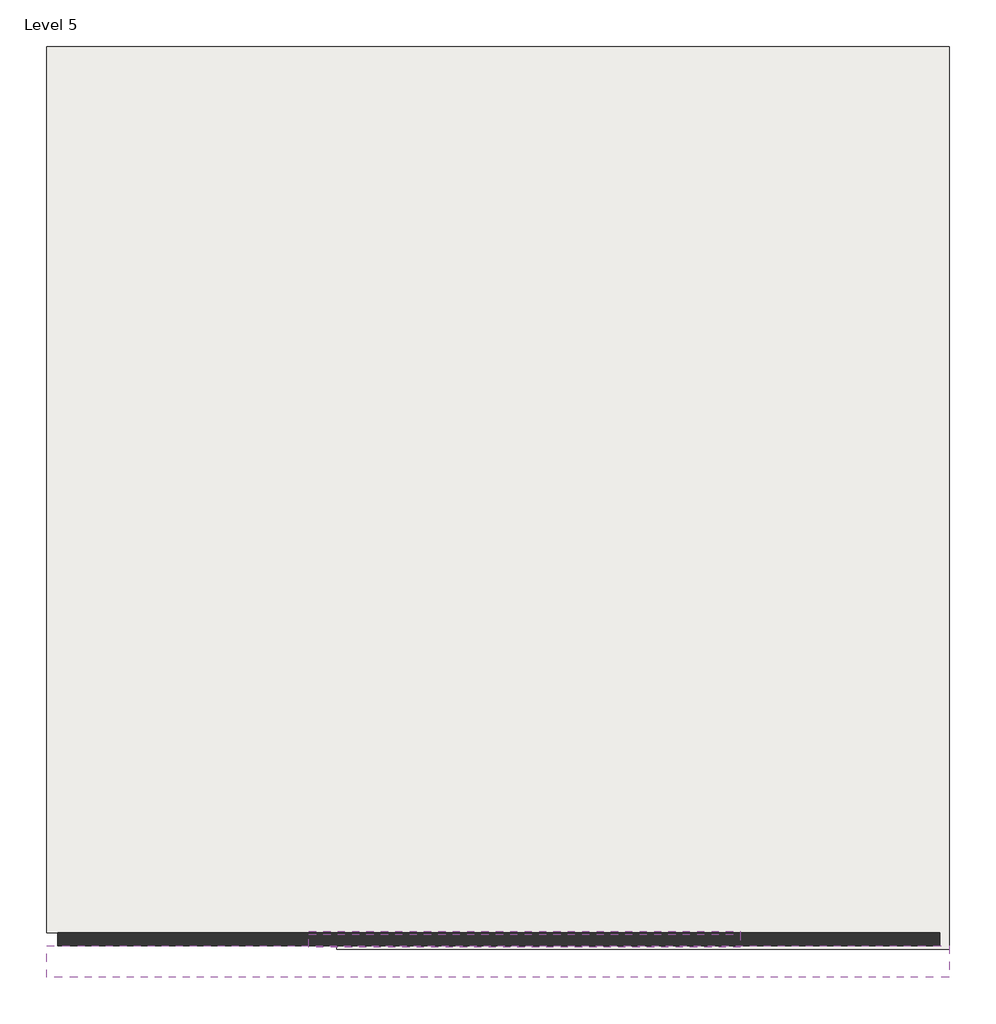
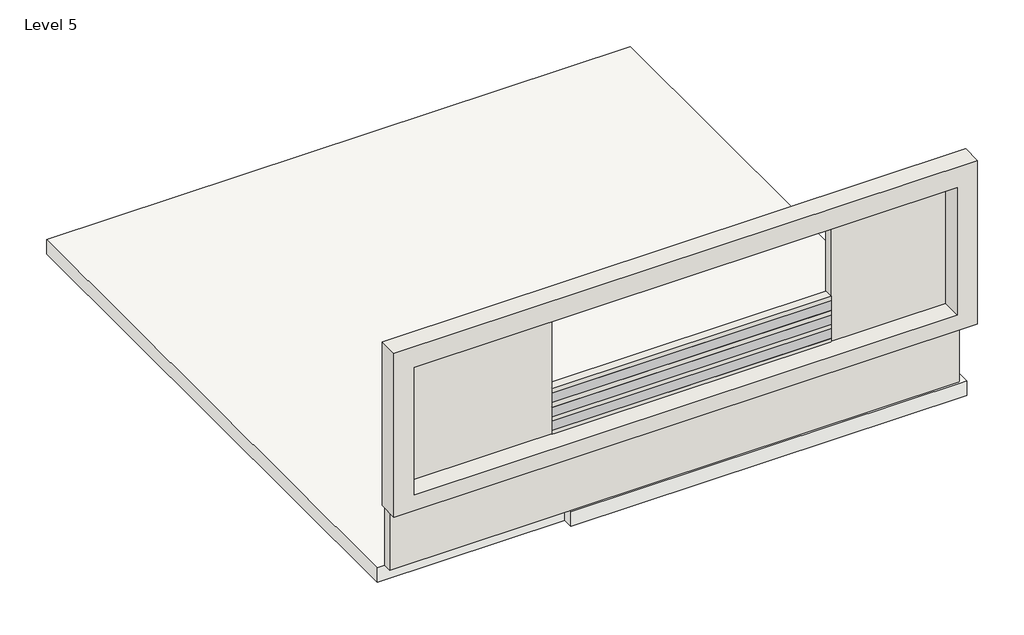
# One storey: 3 proxies, 3 walls, 1 roof.
"""IFC4 building model written with IfcOpenShell, lengths in millimetres."""

from ifc_helpers import new_model, si_unit, frame, origin, place, context, project, spatial, polyline, outline, extrude, faceted_brep, transform, mapped, element, save
from components import walls_4_walls_4_69c7fff0

model = new_model("IFC4")

# Units and contexts
model_context = context("Model", 3, world=origin())
ifc_project = project(units=[si_unit("LENGTHUNIT", "METRE", prefix="MILLI")], contexts=[model_context])

# Site, building, storey
site = spatial("IfcSite", under=ifc_project)
building = spatial("IfcBuilding", under=site)
storey = spatial("IfcBuildingStorey", under=building, Name="Level 5", Elevation=15544.8)

# Proxies
placement = place(None, origin())
element("IfcBuildingElementProxy", 1, Name="Reveal", ObjectType="Reveal", at=placement, inside=storey, context=model_context, shape_type="SweptSolid", body=[
    extrude(outline(polyline([(-6293.9561565, 1484.2485991), (-6293.9561565, 1636.6485991), (-2118.5901764, 1636.6485991), (-2118.5901764, 1484.2485991), (-6293.9561565, 1484.2485991)])), frame((0.0, 0.0, 17589.4520409), z_axis=(0.0, 0.0, 1.0), x_axis=(1.0, 0.0, 0.0)), (0.0, 0.0, 1.0), 152.4),
])
element("IfcBuildingElementProxy", 2, Name="Reveal", ObjectType="Reveal", at=placement, inside=storey, context=model_context, shape_type="SweptSolid", body=[
    extrude(outline(polyline([(-6293.9561565, 1484.2485991), (-6293.9561565, 1636.6485991), (-2118.5901764, 1636.6485991), (-2118.5901764, 1484.2485991), (-6293.9561565, 1484.2485991)])), frame((0.0, 0.0, 17360.8520409), z_axis=(0.0, 0.0, 1.0), x_axis=(1.0, 0.0, 0.0)), (0.0, 0.0, 1.0), 152.4),
])
element("IfcBuildingElementProxy", 3, Name="Reveal", ObjectType="Reveal", at=placement, inside=storey, context=model_context, shape_type="SweptSolid", body=[
    extrude(outline(polyline([(-6293.9561565, 1484.2485991), (-6293.9561565, 1636.6485991), (-2118.5901764, 1636.6485991), (-2118.5901764, 1484.2485991), (-6293.9561565, 1484.2485991)])), frame((0.0, 0.0, 17145.0), z_axis=(0.0, 0.0, 1.0), x_axis=(1.0, 0.0, 0.0)), (0.0, 0.0, 1.0), 152.4),
])

# Roof
element("IfcRoof", 4, ObjectType="Generic - 9\"", at=placement, inside=storey, context=model_context, shape_type="SweptSolid", body=[
    extrude(outline(polyline([(-8833.9561565, 10202.7985991), (-96.3561565, 10202.7985991), (-96.3561565, 1465.1985991), (-6027.2561565, 1465.1985991), (-6027.2561565, 1623.9485991), (-8833.9561565, 1623.9485991), (-8833.9561565, 10202.7985991)])), frame((0.0, 0.0, 15544.8), z_axis=(0.0, 0.0, 1.0), x_axis=(1.0, 0.0, 0.0)), (0.0, 0.0, 1.0), 228.6),
])

# Walls
element("IfcWall", 5, ObjectType="Generic - 5\"", at=placement, inside=storey, context=model_context, shape_type="Brep", body=[
    faceted_brep([(-8724.447025, 1496.6402851, 15773.4), (-190.047025, 1496.6402851, 15773.4), (-190.047025, 1496.6402851, 19202.4), (-2118.5901764, 1496.6402851, 19202.4), (-2118.5901764, 1496.6402851, 17741.8520409), (-2118.5901764, 1496.6402851, 17589.4520409), (-2118.5901764, 1496.6402851, 17513.2520409), (-2118.5901764, 1496.6402851, 17360.8520409), (-2118.5901764, 1496.6402851, 17297.4), (-2118.5901764, 1496.6402851, 17145.0), (-2118.5901764, 1496.6402851, 17087.4973119), (-6293.9561565, 1496.6402851, 17087.4973119), (-6293.9561565, 1496.6402851, 17145.0), (-6293.9561565, 1496.6402851, 17297.4), (-6293.9561565, 1496.6402851, 17360.8520409), (-6293.9561565, 1496.6402851, 17513.2520409), (-6293.9561565, 1496.6402851, 17589.4520409), (-6293.9561565, 1496.6402851, 17741.8520409), (-6293.9561565, 1496.6402851, 19202.4), (-8724.447025, 1496.6402851, 19202.4), (-190.047025, 1623.6402851, 15773.4), (-8724.447025, 1623.6402851, 15773.4), (-8724.447025, 1623.6402851, 19202.4), (-6293.9561565, 1623.6402851, 19202.4), (-6293.9561565, 1623.6402851, 17741.8520409), (-6293.9561565, 1623.6402851, 17589.4520409), (-6293.9561565, 1623.6402851, 17513.2520409), (-6293.9561565, 1623.6402851, 17360.8520409), (-6293.9561565, 1623.6402851, 17297.4), (-6293.9561565, 1623.6402851, 17145.0), (-6293.9561565, 1623.6402851, 17087.4973119), (-2118.5901764, 1623.6402851, 17087.4973119), (-2118.5901764, 1623.6402851, 17145.0), (-2118.5901764, 1623.6402851, 17297.4), (-2118.5901764, 1623.6402851, 17360.8520409), (-2118.5901764, 1623.6402851, 17513.2520409), (-2118.5901764, 1623.6402851, 17589.4520409), (-2118.5901764, 1623.6402851, 17741.8520409), (-2118.5901764, 1623.6402851, 19202.4), (-190.047025, 1623.6402851, 19202.4), (-2118.5901764, 1611.2485991, 17087.4973119), (-6293.9561565, 1611.2485991, 17087.4973119)], [[[0, 1, 2, 3, 4, 5, 6, 7, 8, 9, 10, 11, 12, 13, 14, 15, 16, 17, 18, 19]], [[20, 21, 22, 23, 24, 25, 26, 27, 28, 29, 30, 31, 32, 33, 34, 35, 36, 37, 38, 39]], [[1, 0, 21, 20]], [[2, 1, 20, 39]], [[0, 19, 22, 21]], [[3, 2, 39, 38]], [[3, 38, 37, 36, 35, 34, 33, 32, 31, 40, 10, 9, 8, 7, 6, 5, 4]], [[11, 10, 40, 31, 30, 41]], [[11, 41, 30, 29, 28, 27, 26, 25, 24, 23, 18, 17, 16, 15, 14, 13, 12]], [[19, 18, 23, 22]]]),
])
element("IfcWall", 6, ObjectType="Generic - 5\"", at=placement, inside=storey, context=model_context, shape_type="Brep", body=[
    faceted_brep([(-6293.9561565, 1484.2485991, 17087.4973119), (-2118.5901764, 1484.2485991, 17087.4973119), (-2118.5901764, 1484.2485991, 17145.0), (-6293.9561565, 1484.2485991, 17145.0), (-2118.5901764, 1611.2485991, 17087.4973119), (-6293.9561565, 1611.2485991, 17087.4973119), (-6293.9561565, 1611.2485991, 17145.0), (-2118.5901764, 1611.2485991, 17145.0), (-6293.9561565, 1496.6402851, 17087.4973119), (-2118.5901764, 1496.6402851, 17087.4973119)], [[[0, 1, 2, 3]], [[4, 5, 6, 7]], [[1, 0, 8, 5, 4, 9]], [[1, 9, 4, 7, 2]], [[5, 8, 0, 3, 6]], [[3, 2, 7, 6]]]),
    faceted_brep([(-2118.5901764, 1484.2485991, 17816.0955653), (-6293.9561565, 1484.2485991, 17816.0955653), (-6293.9561565, 1484.2485991, 17741.8520409), (-2118.5901764, 1484.2485991, 17741.8520409), (-6293.9561565, 1611.2485991, 17816.0955653), (-2118.5901764, 1611.2485991, 17816.0955653), (-2118.5901764, 1611.2485991, 17741.8520409), (-6293.9561565, 1611.2485991, 17741.8520409)], [[[0, 1, 2, 3]], [[4, 5, 6, 7]], [[5, 0, 3, 6]], [[1, 0, 5, 4]], [[1, 4, 7, 2]], [[3, 2, 7, 6]]]),
    faceted_brep([(-2118.5901764, 1484.2485991, 17589.4520409), (-6293.9561565, 1484.2485991, 17589.4520409), (-6293.9561565, 1484.2485991, 17513.2520409), (-2118.5901764, 1484.2485991, 17513.2520409), (-6293.9561565, 1611.2485991, 17589.4520409), (-2118.5901764, 1611.2485991, 17589.4520409), (-2118.5901764, 1611.2485991, 17513.2520409), (-6293.9561565, 1611.2485991, 17513.2520409)], [[[0, 1, 2, 3]], [[4, 5, 6, 7]], [[5, 0, 3, 6]], [[1, 4, 7, 2]], [[1, 0, 5, 4]], [[3, 2, 7, 6]]]),
    faceted_brep([(-2118.5901764, 1484.2485991, 17360.8520409), (-6293.9561565, 1484.2485991, 17360.8520409), (-6293.9561565, 1484.2485991, 17297.4), (-2118.5901764, 1484.2485991, 17297.4), (-6293.9561565, 1611.2485991, 17360.8520409), (-2118.5901764, 1611.2485991, 17360.8520409), (-2118.5901764, 1611.2485991, 17297.4), (-6293.9561565, 1611.2485991, 17297.4)], [[[0, 1, 2, 3]], [[4, 5, 6, 7]], [[5, 0, 3, 6]], [[1, 4, 7, 2]], [[1, 0, 5, 4]], [[3, 2, 7, 6]]]),
])
walls_4_walls_4_shape = walls_4_walls_4_69c7fff0(model_context)
element("IfcWall", 7, ObjectType="Walls 4 : Walls 4", at=placement, inside=storey, context=model_context, shape_type="MappedRepresentation", body=[
    mapped(walls_4_walls_4_shape, transform((0.0, 0.0, 0.0), x_axis=(1.0, 0.0, 0.0), y_axis=(0.0, 1.0, 0.0), z_axis=(0.0, 0.0, 1.0))),
])

save(model, "model.ifc")

# Revit data of these elements
# Type "Generic - 9\""
#   Assembly Code = "B1020"
#   Layers, outside or top first: 0' - 9" no material (function 1)
# Type "Generic - 5\""
#   Assembly Code = "B2010"
#   Layers, outside or top first: 0' - 5" no material (function 1)
# Element 4 (IfcRoof, "Generic - 9\"")
#   built-in parameter 1001705 = 51.75 (stored number, unit not read)
#   built-in parameter 1001710 = 33615
#   Phase Created = New Construction
#   Materials on its faces: "Default Roof"
# Element 5 (IfcWall, "Generic - 5\"")
#   built-in parameter 1001111 = 0' - 9"
#   Top Offset = 0' - 0"
#   Base Offset = 0' - 9"
#   wall height = 11' - 3"
#   Phase Created = New Construction
#   Base Constraint = Level 5
#   Top Constraint = Level 6
#   Materials on its faces: "Default Wall"
# Element 6 (IfcWall, "Generic - 5\"")
#   built-in parameter 1001111 = 5' - 0.73611"
#   Top Offset = -4' - 6.57891"
#   Base Offset = 5' - 0.73611"
#   wall height = 2' - 4.68497"
#   Phase Created = New Construction
#   Base Constraint = Level 5
#   Top Constraint = Level 6
#   Materials on its faces: "Default Wall"
# Element 7 (IfcWall, "Walls 4 : Walls 4")
#   Phase Created = New Construction
#   Materials on its faces: "Default Wall"
# Materials
#   "Default Roof": colour RGB 88 101 114, transparency 0
#   "Default Wall": colour RGB 128 128 128, transparency 0
